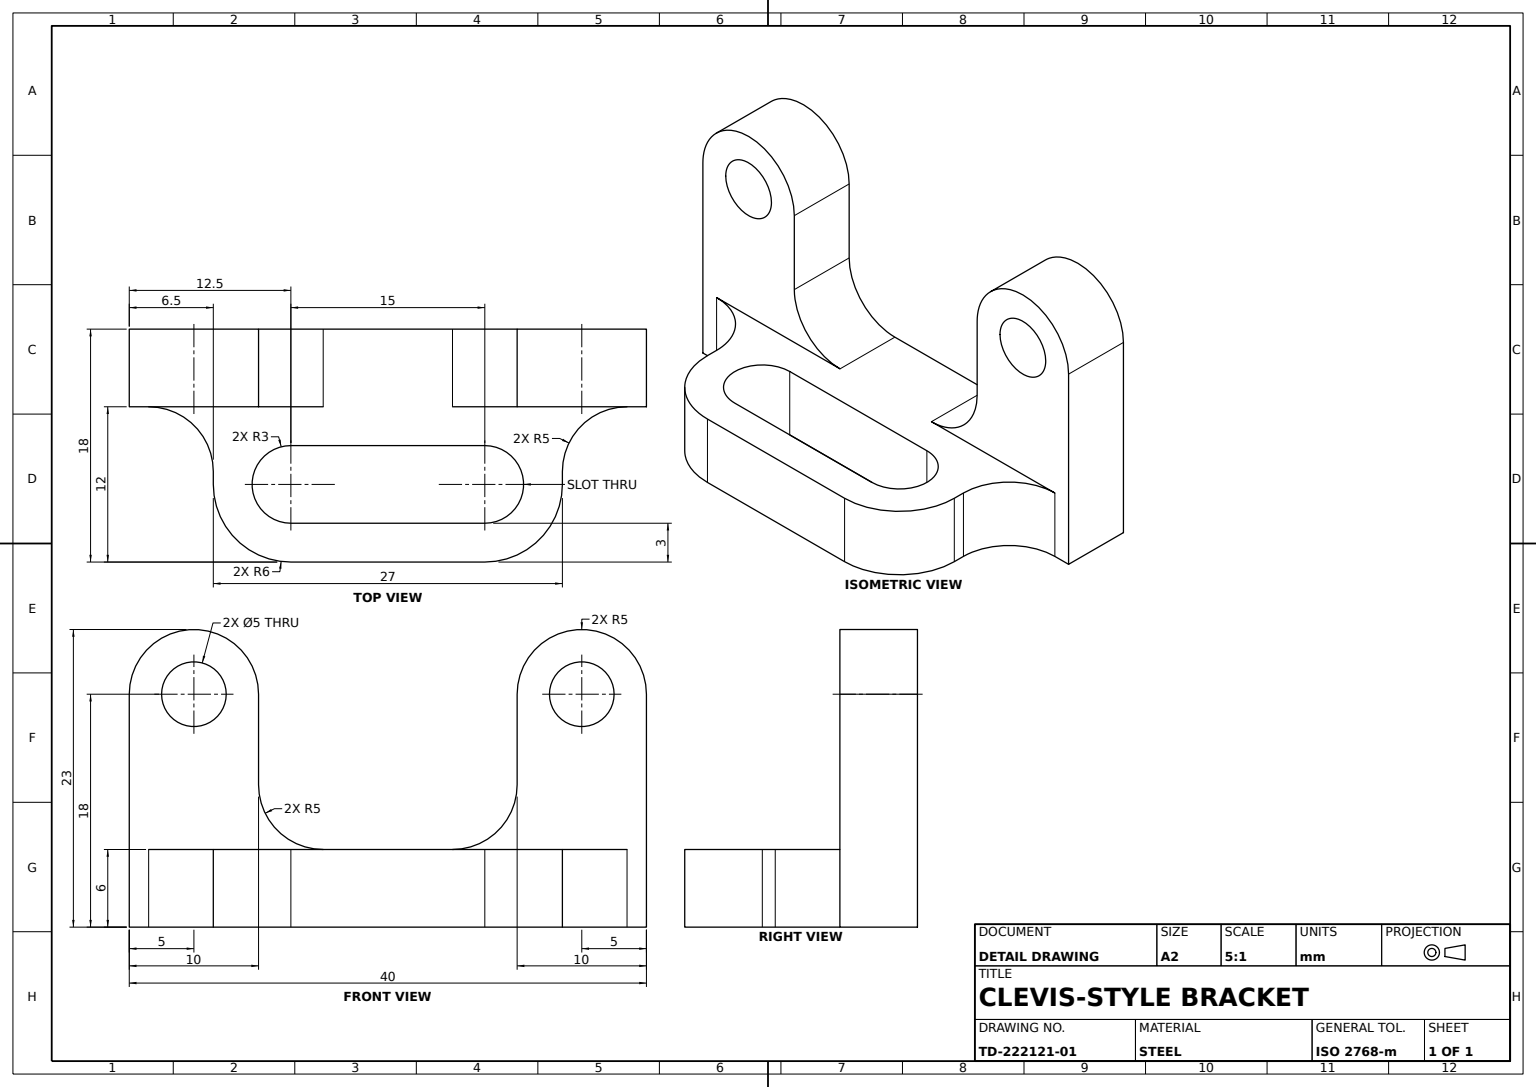
from build123d import *

# Parameters (mm, degrees)
BRACKET_PROFILE_DEPTH     = 6
UPRIGHT_ROUNDS_R5_R       = 5
BASE_PLATE_SKETCH_W       = 27
BASE_PLATE_SKETCH_H       = 6
BASE_PLATE_DEPTH          = 12
BASE_PLATE_ROUNDS_R6_R    = 6
BASE_UPRIGHT_FILLETS_R5_R = 5
BASE_SLOT_DEPTH           = 6
PIVOT_HOLES_SKETCH_R      = 2.5
PIVOT_HOLES_2X_5_DEPTH    = 6


with BuildPart() as part:
    # Bracket Profile Sketch → Bracket Profile (new body)
    with BuildSketch(Plane.XY):
        with BuildLine():
            Line((-20, 0), (20, 0))
            Line((20, 0), (20, 18))
            ThreePointArc((20, 18), (15, 23), (10, 18))
            Line((10, 18), (10, 6))
            Line((10, 6), (-10, 6))
            Line((-10, 6), (-10, 18))
            ThreePointArc((-10, 18), (-15, 23), (-20, 18))
            Line((-20, 18), (-20, 0))
        make_face()
    extrude(amount=BRACKET_PROFILE_DEPTH)

    # Upright Rounds R5
    upright_rounds_r5_edges = [part.edges().sort_by_distance(p)[0] for p in [
        (-10, 6, 3),
        (10, 6, 3),
    ]]
    fillet(upright_rounds_r5_edges, radius=UPRIGHT_ROUNDS_R5_R)

    # Base Plate Sketch → Base Plate (add)
    with BuildSketch(Plane.XY.offset(6)):
        with Locations((0, 3)):
            Rectangle(BASE_PLATE_SKETCH_W, BASE_PLATE_SKETCH_H)
    extrude(amount=BASE_PLATE_DEPTH)

    # Base Plate Rounds R6
    base_plate_rounds_r6_edges = [part.edges().sort_by_distance(p)[0] for p in [
        (-13.5, 3, 18),
        (13.5, 3, 18),
    ]]
    fillet(base_plate_rounds_r6_edges, radius=BASE_PLATE_ROUNDS_R6_R)

    # Base-Upright Fillets R5
    base_upright_fillets_r5_edges = [part.edges().sort_by_distance(p)[0] for p in [
        (-13.5, 3, 6),
        (13.5, 3, 6),
    ]]
    fillet(base_upright_fillets_r5_edges, radius=BASE_UPRIGHT_FILLETS_R5_R)

    # Base Slot Sketch → Base Slot (cut)
    with BuildSketch(Plane(origin=(0, 6, 0), x_dir=(1, 0, 0), z_dir=(0, 1, 0))):
        with BuildLine():
            Line((-7.5, -9), (7.5, -9))
            ThreePointArc((7.5, -9), (10.5, -12), (7.5, -15))
            Line((7.5, -15), (-7.5, -15))
            ThreePointArc((-7.5, -15), (-10.5, -12), (-7.5, -9))
        make_face()
    extrude(amount=-BASE_SLOT_DEPTH, mode=Mode.SUBTRACT)

    # Pivot Holes Sketch → Pivot Holes 2xØ5 (cut)
    with BuildSketch(Plane.XY.offset(6)):
        with Locations((-15, 18)):
            Circle(PIVOT_HOLES_SKETCH_R)
        with Locations((15, 18)):
            Circle(PIVOT_HOLES_SKETCH_R)
    extrude(amount=-PIVOT_HOLES_2X_5_DEPTH, mode=Mode.SUBTRACT)


solid = part.part
